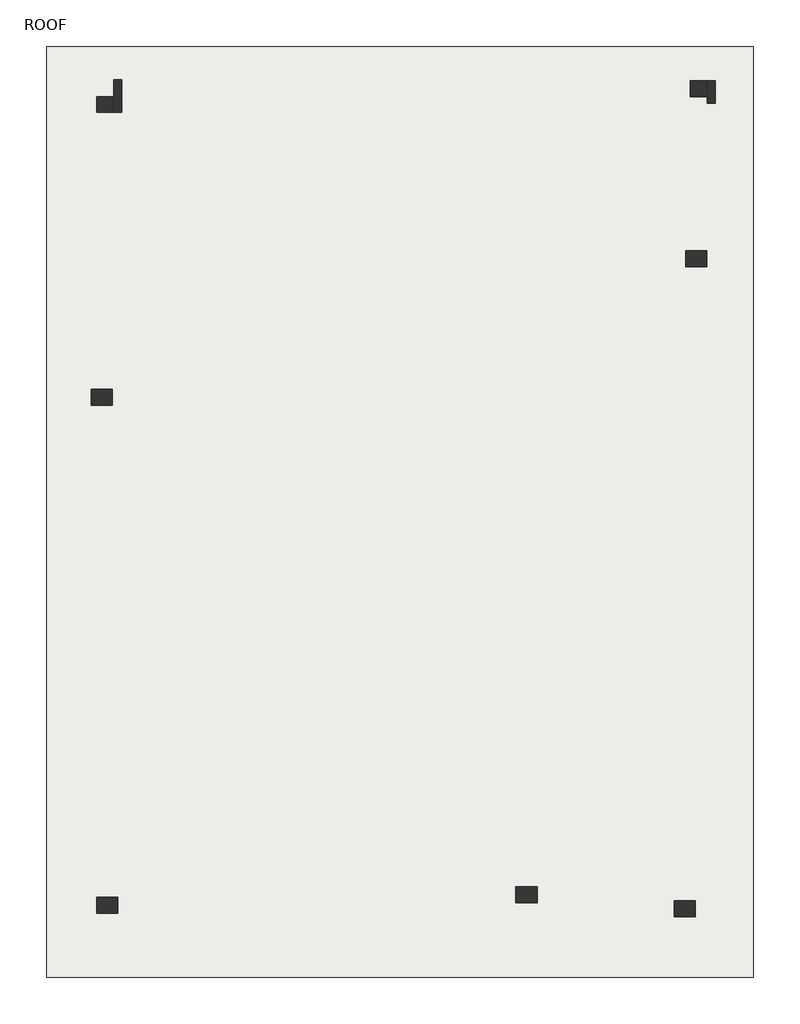
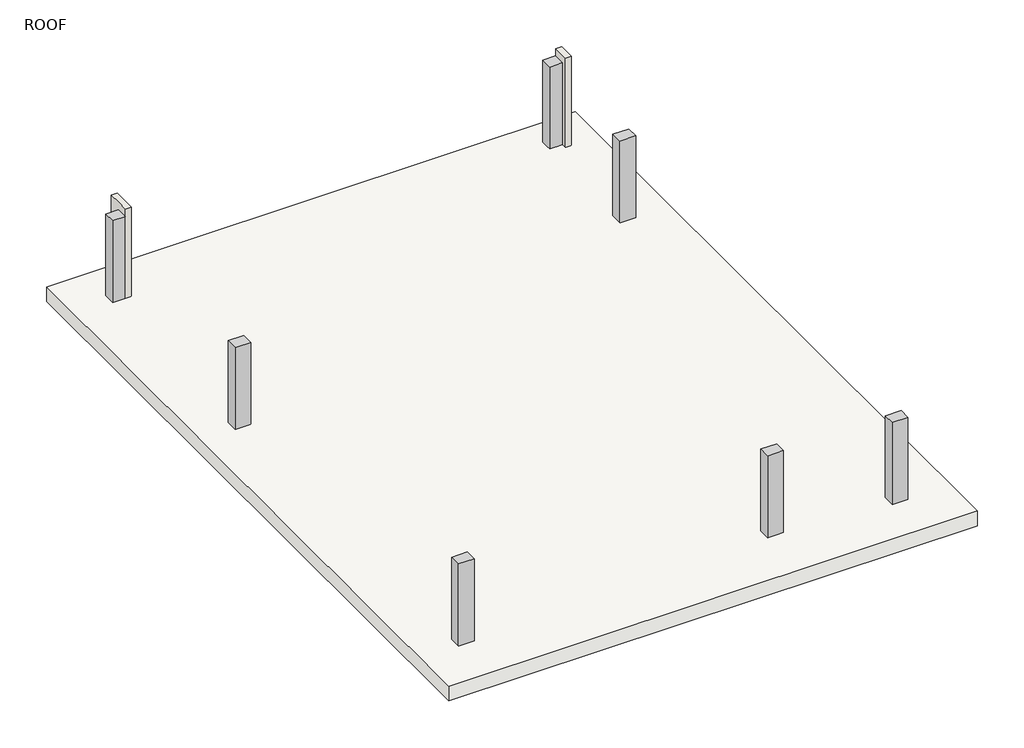
# One storey: 7 columns, 2 walls, 1 slab.
"""IFC4 building model written with IfcOpenShell, lengths in millimetres."""

from ifc_helpers import new_model, si_unit, frame, origin, place, context, project, spatial, polyline, outline, extrude, faceted_brep, element, save

model = new_model("IFC4")

# Units and contexts
model_context = context("Model", 3, world=origin())
ifc_project = project(units=[si_unit("LENGTHUNIT", "METRE", prefix="MILLI")], contexts=[model_context])

# Site, building, storey
site = spatial("IfcSite", under=ifc_project)
building = spatial("IfcBuilding", under=site)
storey = spatial("IfcBuildingStorey", under=building, Name="ROOF", Elevation=6400.8)

# Columns
placement = place(None, origin())
element("IfcColumn", 1, ObjectType="Rectangular Column : 1'9\"", at=placement, inside=storey, context=model_context, shape_type="SweptSolid", body=[
    extrude(outline(polyline([(10828.4334712, 491.3450307), (10828.4334712, 262.7450307), (10523.6334712, 262.7450307), (10523.6334712, 491.3450307), (10828.4334712, 491.3450307)])), frame((0.0, 0.0, 6400.8), z_axis=(0.0, 0.0, 1.0), x_axis=(1.0, 0.0, 0.0)), (0.0, 0.0, 1.0), 1676.4),
])
element("IfcColumn", 2, ObjectType="Rectangular Column : 1'9\"", at=placement, inside=storey, context=model_context, shape_type="SweptSolid", body=[
    extrude(outline(polyline([(8542.4334712, 694.5450307), (8542.4334712, 465.9450307), (8237.6334712, 465.9450307), (8237.6334712, 694.5450307), (8542.4334712, 694.5450307)])), frame((0.0, 0.0, 6400.8), z_axis=(0.0, 0.0, 1.0), x_axis=(1.0, 0.0, 0.0)), (0.0, 0.0, 1.0), 1676.4),
])
element("IfcColumn", 3, ObjectType="Rectangular Column : 1'9\"", at=placement, inside=storey, context=model_context, shape_type="SweptSolid", body=[
    extrude(outline(polyline([(2484.5334712, 542.1450307), (2484.5334712, 313.5450307), (2179.7334712, 313.5450307), (2179.7334712, 542.1450307), (2484.5334712, 542.1450307)])), frame((0.0, 0.0, 6400.8), z_axis=(0.0, 0.0, 1.0), x_axis=(1.0, 0.0, 0.0)), (0.0, 0.0, 1.0), 1676.4),
])
element("IfcColumn", 4, ObjectType="Rectangular Column : 1'9\"", at=placement, inside=storey, context=model_context, shape_type="SweptSolid", body=[
    extrude(outline(polyline([(2408.3334712, 7882.7450307), (2408.3334712, 7654.1450307), (2103.5334712, 7654.1450307), (2103.5334712, 7882.7450307), (2408.3334712, 7882.7450307)])), frame((0.0, 0.0, 6400.8), z_axis=(0.0, 0.0, 1.0), x_axis=(1.0, 0.0, 0.0)), (0.0, 0.0, 1.0), 1676.4),
])
element("IfcColumn", 5, ObjectType="Rectangular Column : 1'9\"", at=placement, inside=storey, context=model_context, shape_type="SweptSolid", body=[
    extrude(outline(polyline([(2179.7334712, 11883.2450307), (2179.7334712, 12111.8450307), (2427.3834712, 12111.8450307), (2427.3834712, 11883.2450307), (2179.7334712, 11883.2450307)])), frame((0.0, 0.0, 6400.8), z_axis=(0.0, 0.0, 1.0), x_axis=(1.0, 0.0, 0.0)), (0.0, 0.0, 1.0), 1676.4),
])
element("IfcColumn", 6, ObjectType="Rectangular Column : 1'9\"", at=placement, inside=storey, context=model_context, shape_type="SweptSolid", body=[
    extrude(outline(polyline([(10752.2334712, 12111.8450307), (10752.2334712, 12340.4450307), (10999.8834712, 12340.4450307), (10999.8834712, 12111.8450307), (10752.2334712, 12111.8450307)])), frame((0.0, 0.0, 6400.8), z_axis=(0.0, 0.0, 1.0), x_axis=(1.0, 0.0, 0.0)), (0.0, 0.0, 1.0), 1676.4),
])
element("IfcColumn", 7, ObjectType="Rectangular Column : 1'9\"", at=placement, inside=storey, context=model_context, shape_type="SweptSolid", body=[
    extrude(outline(polyline([(10993.5334712, 9882.9950307), (10993.5334712, 9654.3950307), (10688.7334712, 9654.3950307), (10688.7334712, 9882.9950307), (10993.5334712, 9882.9950307)])), frame((0.0, 0.0, 6400.8), z_axis=(0.0, 0.0, 1.0), x_axis=(1.0, 0.0, 0.0)), (0.0, 0.0, 1.0), 1676.4),
])

# Slab
element("IfcSlab", 8, ObjectType="Generic - 12\"", at=placement, inside=storey, context=model_context, shape_type="SweptSolid", body=[
    extrude(outline(polyline([(11666.6334712, 12835.7450307), (11666.6334712, -613.5549693), (1455.8334712, -613.5549693), (1455.8334712, 12835.7450307), (11666.6334712, 12835.7450307)])), frame((0.0, 0.0, 6096.0), z_axis=(0.0, 0.0, 1.0), x_axis=(1.0, 0.0, 0.0)), (0.0, 0.0, 1.0), 304.8),
])

# Walls
element("IfcWall", 9, ObjectType="Generic - 4.5\"", at=placement, inside=storey, context=model_context, shape_type="Brep", body=[
    faceted_brep([(2427.3834712, 12356.5156894, 6400.8), (2427.3834712, 12111.8450307, 6400.8), (2427.3834712, 11883.2450307, 6400.8), (2427.3834712, 11883.2450307, 8077.2), (2427.3834712, 11883.2450307, 8229.6), (2427.3834712, 12111.8450307, 8229.6), (2427.3834712, 12356.5156894, 8229.6), (2541.6834712, 12356.5156894, 6400.8), (2541.6834712, 12356.5156894, 8229.6), (2541.6834712, 11883.2450307, 8229.6), (2541.6834712, 11883.2450307, 6400.8)], [[[0, 1, 2, 3, 4, 5, 6]], [[7, 8, 9, 10]], [[2, 1, 0, 7, 10]], [[4, 3, 2, 10, 9]], [[6, 5, 4, 9, 8]], [[0, 6, 8, 7]]]),
])
element("IfcWall", 10, ObjectType="Generic - 4.5\"", at=placement, inside=storey, context=model_context, shape_type="Brep", body=[
    faceted_brep([(11114.1834712, 12017.602252, 6400.8), (11114.1834712, 12340.4450307, 6400.8), (11114.1834712, 12340.4450307, 8229.6), (11114.1834712, 12017.602252, 8229.6), (10999.8834712, 12017.602252, 6400.8), (10999.8834712, 12017.602252, 8229.6), (10999.8834712, 12111.8450307, 8229.6), (10999.8834712, 12340.4450307, 8229.6), (10999.8834712, 12340.4450307, 8077.2), (10999.8834712, 12340.4450307, 6400.8), (10999.8834712, 12111.8450307, 6400.8)], [[[0, 1, 2, 3]], [[4, 5, 6, 7, 8, 9, 10]], [[1, 0, 4, 10, 9]], [[2, 1, 9, 8, 7]], [[3, 2, 7, 6, 5]], [[0, 3, 5, 4]]]),
])

save(model, "model.ifc")

# Revit data of these elements
# Type "Rectangular Column : 1'9\""
#   Assembly Code = "B1010200"
#   Depth = 0' - 9"
#   Offset Base = 0' - 0"
#   Offset Top = 0' - 0"
#   Width = 1' - 0"
#   Material = none
# Type "Generic - 12\""
#   Assembly Code = "B1010"
#   Function = 0
#   Layers, outside or top first: 1' - 0" no material (function 1)
# Type "Generic - 4.5\""
#   Assembly Code = "B2010"
#   Layers, outside or top first: 0' - 4 1/2" no material (function 1)
# Elements 1, 2, 3, 4, 7 (IfcColumn, "Rectangular Column : 1'9\"")
#   Phase Created = New Construction
# Elements 5, 6 (IfcColumn, "Rectangular Column : 1'9\"")
#   Phase Created = New Construction
#   Materials on its faces: "Default Wall"
# Element 8 (IfcSlab, "Generic - 12\"")
#   Height Offset From Level = 0' - 0"
#   Phase Created = New Construction
#   Materials on its faces: "Default Floor"
# Elements 9, 10 (IfcWall, "Generic - 4.5\"")
#   Top Offset = 0' - 0"
#   Base Offset = 0' - 0"
#   wall height = 6' - 0"
#   Phase Created = New Construction
#   Base Constraint = ROOF
#   Top Constraint = PARAPET WALL
#   Materials on its faces: "Default Wall"
# Materials
#   "Default Wall": colour RGB 128 128 128, transparency 0, Cost = 0
#   "Default Floor": colour RGB 128 128 128, transparency 0, Cost = 0
